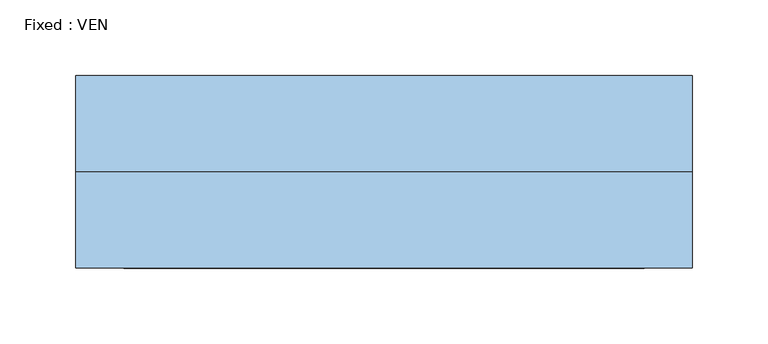
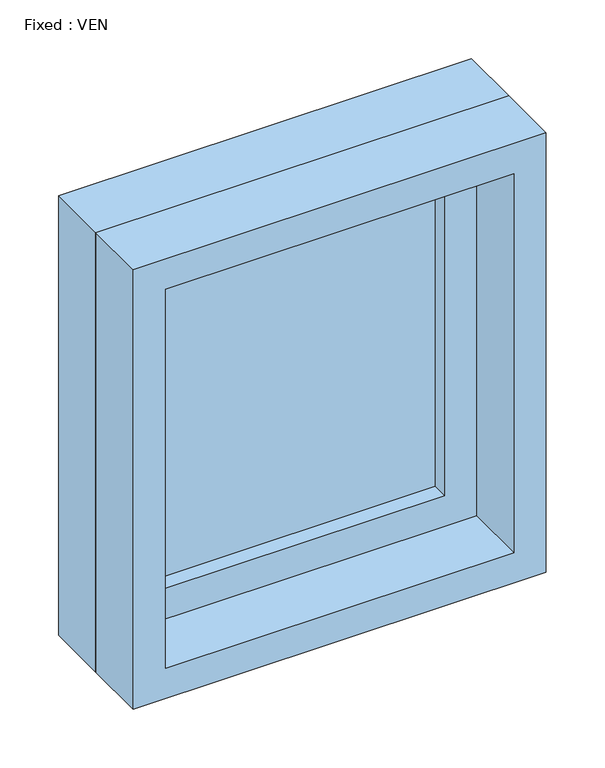
"""IFC4 building model written with IfcOpenShell, lengths in millimetres: window geometry, Fixed : VEN."""

from ifc_helpers import new_model, si_unit, frame, origin, place, context, project, spatial, polyline, outline, extrude, source, transform, mapped, element, save


def fixed_ven_0bde2124(model_context):
    return source(origin(), model_context, "Body", "SweptSolid", [
        extrude(outline(polyline([(101.6, 15.875), (-177.8, 15.875), (-177.8, 28.575), (101.6, 28.575), (101.6, 15.875)])), frame((0.0, 0.0, 977.9), z_axis=(0.0, 0.0, 1.0), x_axis=(1.0, 0.0, 0.0)), (0.0, 0.0, 1.0), 330.2),
        extrude(outline(polyline([(1352.55, -222.25), (933.45, -222.25), (933.45, 146.05), (1352.55, 146.05), (1352.55, -222.25)]), holes=[polyline([(1308.1, -177.8), (1308.1, 101.6), (977.9, 101.6), (977.9, -177.8), (1308.1, -177.8)])]), frame((0.0, 0.0, 0.0), z_axis=(0.0, 1.0, 0.0), x_axis=(0.0, 0.0, 1.0)), (0.0, 0.0, 1.0), 44.45),
        extrude(outline(polyline([(1371.6, -241.3), (914.4, -241.3), (914.4, 165.1), (1371.6, 165.1), (1371.6, -241.3)]), holes=[polyline([(1339.85, -209.55), (1339.85, 133.35), (946.15, 133.35), (946.15, -209.55), (1339.85, -209.55)])]), frame((0.0, -63.5, 0.0), z_axis=(0.0, 1.0, 0.0), x_axis=(0.0, 0.0, 1.0)), (0.0, 0.0, 1.0), 63.5),
        extrude(outline(polyline([(1371.6, 165.1), (1371.6, -241.3), (914.4, -241.3), (914.4, 165.1), (1371.6, 165.1)]), holes=[polyline([(1352.55, 146.05), (933.45, 146.05), (933.45, -222.25), (1352.55, -222.25), (1352.55, 146.05)])]), frame((0.0, 0.0, 0.0), z_axis=(0.0, 1.0, 0.0), x_axis=(0.0, 0.0, 1.0)), (0.0, 0.0, 1.0), 63.5),
    ])


if __name__ == "__main__":
    model = new_model("IFC4")
    model_context = context("Model", 3, world=origin())
    ifc_project = project(units=[si_unit("LENGTHUNIT", "METRE", prefix="MILLI")], contexts=[model_context])
    site = spatial("IfcSite", under=ifc_project)
    building = spatial("IfcBuilding", under=site)
    placement = place(None, origin())
    fixed_ven_shape = fixed_ven_0bde2124(model_context)
    element("IfcWindow", 1, ObjectType="Fixed : VEN", at=placement, inside=building, context=model_context, shape_type="MappedRepresentation", body=[
        mapped(fixed_ven_shape, transform((0.0, 0.0, 0.0), x_axis=(1.0, 0.0, 0.0), y_axis=(0.0, 1.0, 0.0), z_axis=(0.0, 0.0, 1.0))),
    ])
    save(model, "model.ifc")

# Revit data of these elements
# Type "Fixed : VEN"
#   Type Mark = "19"
#   Construction Type Id = "GSP4R"
#   Assembly Code = "B2020100"
#   Analytic Construction = "1/8 in Pilkington single glazing"
#   Visual Light Transmittance = 0.9
#   Solar Heat Gain Coefficient = 0.78
#   Heat Transfer Coefficient (U) = 0.6496 BTU/(h·ft²·°F)
#   Height = 1' - 6"
#   Default Sill Height = 3' - 0"
#   Width = 1' - 4"
#   Window Inset = 0' - 0 3/4"
#   Define Thermal Properties by = 1
#   Glass Pane Material = Glass
#   Sash Material = Sash
#   Wall Closure = (empty or 0)
# Element 1 (IfcWindow, "Fixed : VEN")
#   Materials on its faces: "Sash", "Glass"
# Materials
#   "Glass": class "Glass", colour RGB 0 128 192, transparency 0.75, Description = "Soda Lime Glass", Cost = 0
#   "Sash": class "Wood", colour RGB 224 178 126, transparency 0, Cost = 0
